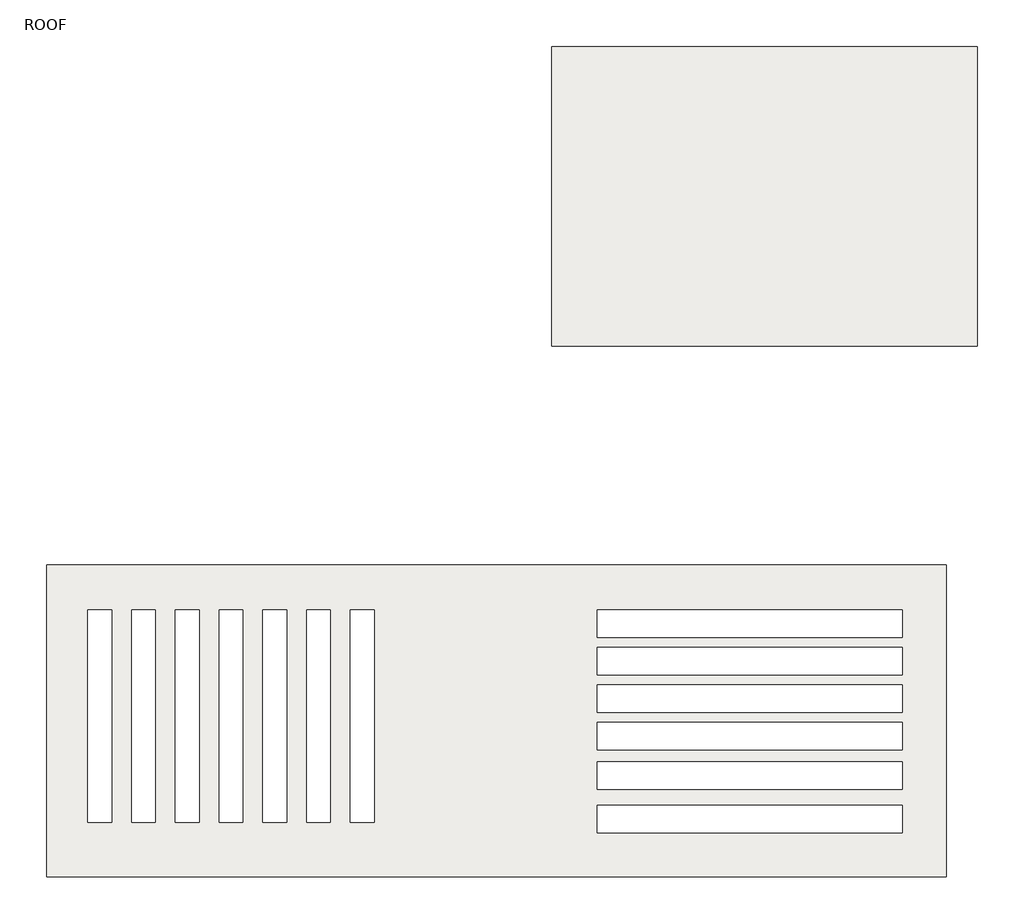
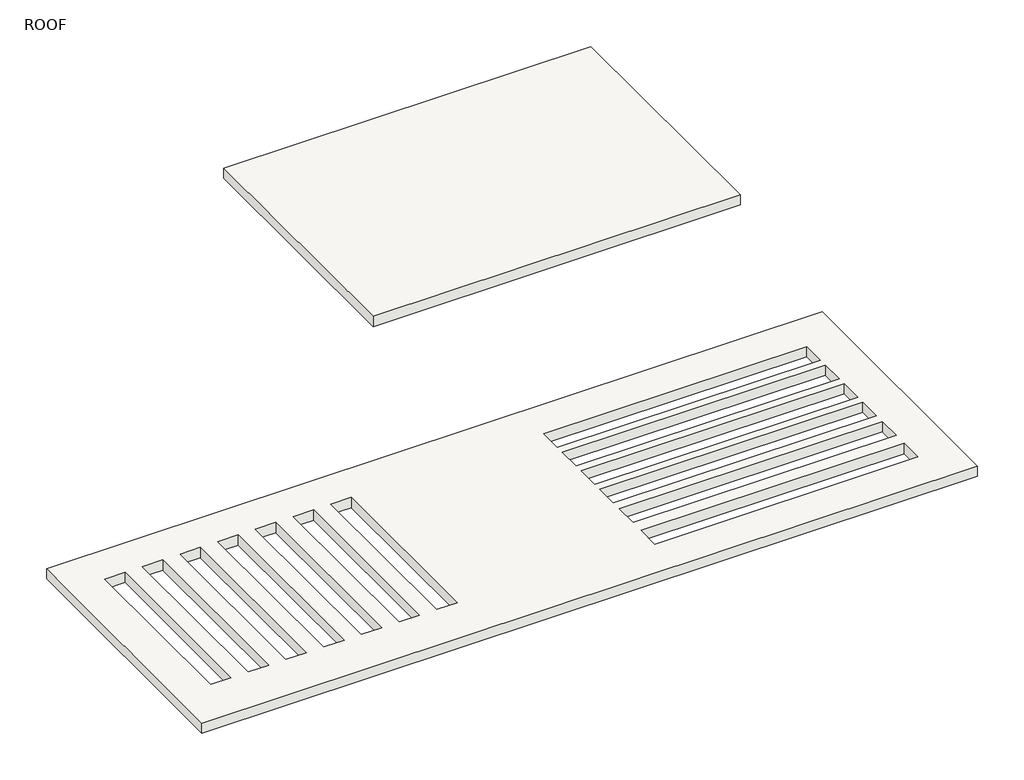
# One storey: 2 slabs.
"""IFC4 building model written with IfcOpenShell, lengths in millimetres."""

from ifc_helpers import new_model, si_unit, frame, origin, place, context, project, spatial, polyline, outline, extrude, element, save

model = new_model("IFC4")

# Units and contexts
model_context = context("Model", 3, world=origin())
ifc_project = project(units=[si_unit("LENGTHUNIT", "METRE", prefix="MILLI")], contexts=[model_context])

# Site, building, storey
site = spatial("IfcSite", under=ifc_project)
building = spatial("IfcBuilding", under=site)
storey = spatial("IfcBuildingStorey", under=building, Name="ROOF", Elevation=12801.6)

# Slabs
placement = place(None, origin())
element("IfcSlab", 1, ObjectType="6\"", at=placement, inside=storey, context=model_context, shape_type="SweptSolid", body=[
    extrude(outline(polyline([(4585.3134019, 2315.1787587), (4585.3134019, -1342.4212413), (-608.948343, -1342.4212413), (-608.948343, 2315.1787587), (4585.3134019, 2315.1787587)])), frame((0.0, 0.0, 12649.2), z_axis=(0.0, 0.0, 1.0), x_axis=(1.0, 0.0, 0.0)), (0.0, 0.0, 1.0), 152.4),
])
element("IfcSlab", 2, ObjectType="6\"", at=placement, inside=storey, context=model_context, shape_type="SweptSolid", body=[
    extrude(outline(polyline([(4204.3134019, -4009.4212413), (4204.3134019, -7819.4212413), (-6768.4865981, -7819.4212413), (-6768.4865981, -4009.4212413), (4204.3134019, -4009.4212413)]), holes=[polyline([(-5974.2886947, -4558.6819233), (-6262.9461303, -4558.6819233), (-6262.9461303, -7154.479328), (-5974.2886947, -7154.479328), (-5974.2886947, -4558.6819233)]), polyline([(-5440.8886947, -4558.6819233), (-5729.5461303, -4558.6819233), (-5729.5461303, -7154.479328), (-5440.8886947, -7154.479328), (-5440.8886947, -4558.6819233)]), polyline([(-4907.4886947, -4558.6819233), (-5196.1461303, -4558.6819233), (-5196.1461303, -7154.479328), (-4907.4886947, -7154.479328), (-4907.4886947, -4558.6819233)]), polyline([(-4374.0886947, -4558.6819233), (-4662.7461303, -4558.6819233), (-4662.7461303, -7154.479328), (-4374.0886947, -7154.479328), (-4374.0886947, -4558.6819233)]), polyline([(-3840.6886947, -4558.6819233), (-4129.3461303, -4558.6819233), (-4129.3461303, -7154.479328), (-3840.6886947, -7154.479328), (-3840.6886947, -4558.6819233)]), polyline([(3670.9134019, -4558.6819233), (-50.1865981, -4558.6819233), (-50.1865981, -4893.298216), (3670.9134019, -4893.298216), (3670.9134019, -4558.6819233)]), polyline([(3670.9134019, -5015.8819233), (-50.1865981, -5015.8819233), (-50.1865981, -5350.498216), (3670.9134019, -5350.498216), (3670.9134019, -5015.8819233)]), polyline([(3670.9134019, -5473.0819233), (-50.1865981, -5473.0819233), (-50.1865981, -5807.698216), (3670.9134019, -5807.698216), (3670.9134019, -5473.0819233)]), polyline([(3670.9134019, -5930.2819233), (-50.1865981, -5930.2819233), (-50.1865981, -6264.898216), (3670.9134019, -6264.898216), (3670.9134019, -5930.2819233)]), polyline([(3670.9134019, -6946.2819233), (-50.1865981, -6946.2819233), (-50.1865981, -7280.898216), (3670.9134019, -7280.898216), (3670.9134019, -6946.2819233)]), polyline([(3670.9134019, -6412.8819233), (-50.1865981, -6412.8819233), (-50.1865981, -6747.498216), (3670.9134019, -6747.498216), (3670.9134019, -6412.8819233)]), polyline([(-3307.2886947, -4558.6819233), (-3595.9461303, -4558.6819233), (-3595.9461303, -7154.479328), (-3307.2886947, -7154.479328), (-3307.2886947, -4558.6819233)]), polyline([(-2773.8886947, -4558.6819233), (-3062.5461303, -4558.6819233), (-3062.5461303, -7154.479328), (-2773.8886947, -7154.479328), (-2773.8886947, -4558.6819233)])]), frame((0.0, 0.0, 12649.2), z_axis=(0.0, 0.0, 1.0), x_axis=(1.0, 0.0, 0.0)), (0.0, 0.0, 1.0), 152.4),
])

save(model, "model.ifc")

# Revit data of these elements
# Type "6\""
#   Assembly Code = "B1010"
#   Function = 0
#   Layers, outside or top first: 0' - 6" no material (function 1)
# Elements 1, 2 (IfcSlab, "6\"")
#   Height Offset From Level = 0' - 0"
#   Phase Created = New Construction
#   Materials on its faces: "Default Floor"
# Materials
#   "Default Floor": colour RGB 128 128 128, transparency 0, Cost = 0
